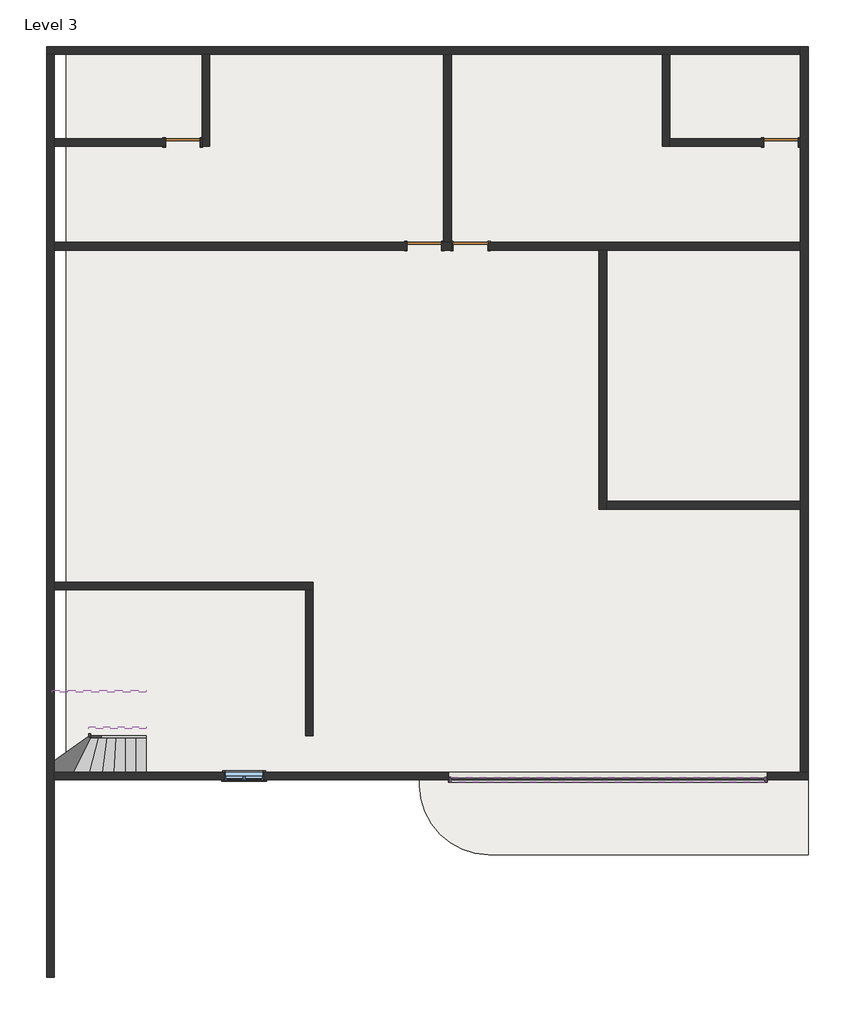
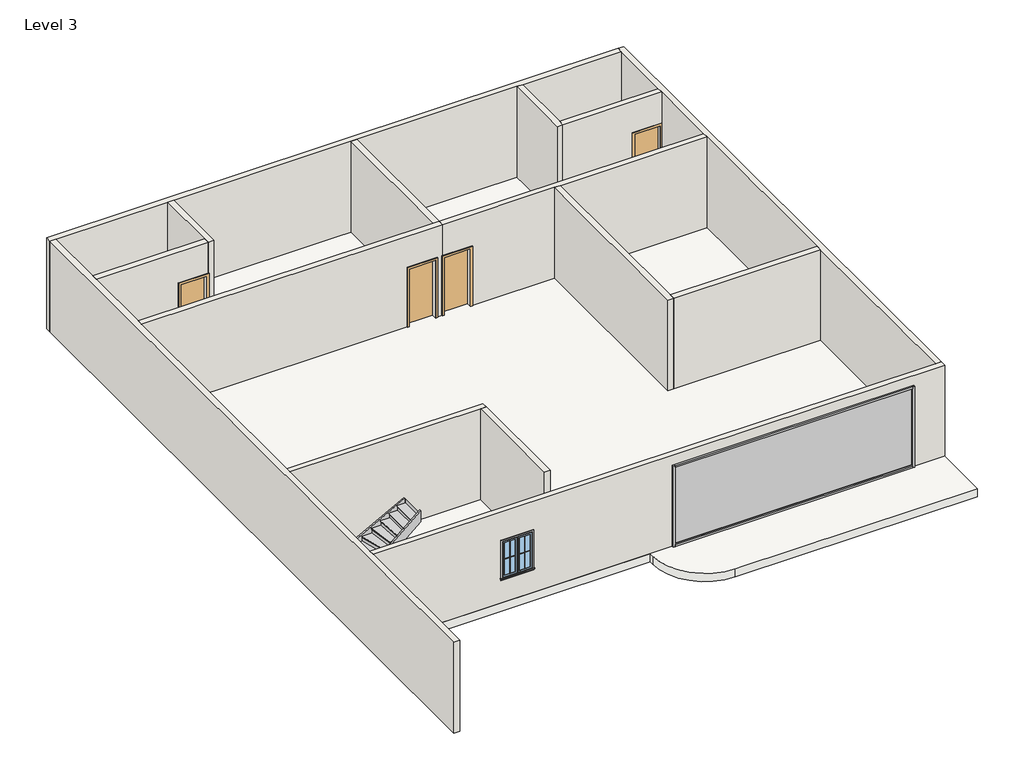
# One storey, incomplete: 15 walls, 12 members, 4 doors, 4 proxies, 1 plate, 1 slab, 1 stair flight, 1 window.
"""IFC4 building model written with IfcOpenShell, lengths in millimetres."""

from ifc_helpers import new_model, si_unit, point, frame, frame_2d, origin, place, context, project, spatial, polyline, circle_curve, trimmed, segment, composite_curve, outline, extrude, faceted_brep, transform, mapped, element, save
from components import muntin_pattern_2x2_muntin_pattern_2x2_88bf7f41, muntin_pattern_2x2_muntin_pattern_2x2_3dfd0a47, trim_window_exterior_flat_with_sill_4930676f, trim_window_interior_flat_picture_frame_dd064338, door_54dd4da4, door_719f80de, member_56b0c076, member_6ded9322, system_panel_glazed_f36121af, stair_flight_a924437b, window_0de3df1e

model = new_model("IFC4")

# Units and contexts
model_context = context("Model", 3, world=origin())
ifc_project = project(units=[si_unit("LENGTHUNIT", "METRE", prefix="MILLI")], contexts=[model_context])

# Site, building, storey
site = spatial("IfcSite", under=ifc_project)
building = spatial("IfcBuilding", under=site)
storey = spatial("IfcBuildingStorey", under=building, Name="Level 3", Elevation=6705.6)

# Proxies
placement = place(None, origin())
muntin_pattern_2x2_muntin_pattern_2x2_shape = muntin_pattern_2x2_muntin_pattern_2x2_88bf7f41(model_context)
element("IfcBuildingElementProxy", 1, Name="Muntin Pattern_2x2 : Muntin Pattern_2x2", ObjectType="Muntin Pattern_2x2 : Muntin Pattern_2x2", at=placement, inside=storey, context=model_context, shape_type="MappedRepresentation", body=[
    mapped(muntin_pattern_2x2_muntin_pattern_2x2_shape, transform((-4862.2306824, -10314.185779, 7689.85), x_axis=(-1.0, 0.0, 0.0), y_axis=(0.0, -1.0, 0.0), z_axis=(0.0, 0.0, 1.0))),
])
muntin_pattern_2x2_muntin_pattern_2x2_2_shape = muntin_pattern_2x2_muntin_pattern_2x2_3dfd0a47(model_context)
element("IfcBuildingElementProxy", 2, Name="Muntin Pattern_2x2 : Muntin Pattern_2x2", ObjectType="Muntin Pattern_2x2 : Muntin Pattern_2x2", at=placement, inside=storey, context=model_context, shape_type="MappedRepresentation", body=[
    mapped(muntin_pattern_2x2_muntin_pattern_2x2_2_shape, transform((-5379.7556824, -10314.185779, 7689.85), x_axis=(1.0, 0.0, 0.0), y_axis=(0.0, 1.0, 0.0), z_axis=(0.0, 0.0, 1.0))),
])
trim_window_exterior_flat_with_sill_shape = trim_window_exterior_flat_with_sill_4930676f(model_context)
element("IfcBuildingElementProxy", 3, Name="Trim-Window-Exterior-Flat : with Sill", ObjectType="Trim-Window-Exterior-Flat : with Sill", at=placement, inside=storey, context=model_context, shape_type="MappedRepresentation", body=[
    mapped(trim_window_exterior_flat_with_sill_shape, transform((-5120.9931824, -10323.710779, 8966.2), x_axis=(1.0, 0.0, 0.0), y_axis=(0.0, 0.0, 1.0), z_axis=(0.0, -1.0, 0.0))),
])
trim_window_interior_flat_picture_frame_shape = trim_window_interior_flat_picture_frame_dd064338(model_context)
element("IfcBuildingElementProxy", 4, Name="Trim-Window-Interior-Flat : Picture Frame", ObjectType="Trim-Window-Interior-Flat : Picture Frame", at=placement, inside=storey, context=model_context, shape_type="MappedRepresentation", body=[
    mapped(trim_window_interior_flat_picture_frame_shape, transform((-5120.9931824, -10120.510779, 8966.2), x_axis=(-1.0, 0.0, 0.0), y_axis=(0.0, 0.0, 1.0), z_axis=(0.0, 1.0, 0.0))),
])

# Doors
door_shape = door_54dd4da4(model_context)
element("IfcDoor", 5, ObjectType="Single-Flush : 36\" x 84\"", at=placement, inside=storey, context=model_context, shape_type="MappedRepresentation", body=[
    mapped(door_shape, transform((-345.7931824, 3798.689221, 6705.6), x_axis=(1.0, 0.0, 0.0), y_axis=(0.0, 1.0, 0.0), z_axis=(0.0, 0.0, 1.0))),
])
element("IfcDoor", 6, ObjectType="Single-Flush : 36\" x 84\"", at=placement, inside=storey, context=model_context, shape_type="MappedRepresentation", body=[
    mapped(door_shape, transform((-6746.5931824, 6541.889221, 6705.6), x_axis=(1.0, 0.0, 0.0), y_axis=(0.0, 1.0, 0.0), z_axis=(0.0, 0.0, 1.0))),
])
door_2_shape = door_719f80de(model_context)
element("IfcDoor", 7, ObjectType="Single-Flush : 36\" x 84\"", at=placement, inside=storey, context=model_context, shape_type="MappedRepresentation", body=[
    mapped(door_2_shape, transform((873.4068176, 3798.689221, 6705.6), x_axis=(-1.0, 0.0, 0.0), y_axis=(0.0, -1.0, 0.0), z_axis=(0.0, 0.0, 1.0))),
])
element("IfcDoor", 8, ObjectType="Single-Flush : 36\" x 84\"", at=placement, inside=storey, context=model_context, shape_type="MappedRepresentation", body=[
    mapped(door_2_shape, transform((9103.0068176, 6541.889221, 6705.6), x_axis=(-1.0, 0.0, 0.0), y_axis=(0.0, -1.0, 0.0), z_axis=(0.0, 0.0, 1.0))),
])

# Members
member_shape = member_56b0c076(model_context)
element("IfcMember", 9, ObjectType="Rectangular Mullion : 2.5\" x 5\" rectangular", at=placement, inside=storey, context=model_context, shape_type="MappedRepresentation", body=[
    mapped(member_shape, transform((296.6565845, -10323.710779, 9700.1946513), x_axis=(-1.0, 0.0, 0.0), y_axis=(0.0, -1.0, 0.0), z_axis=(0.0, 0.0, 1.0))),
])
member_2_shape = member_6ded9322(model_context)
element("IfcMember", 10, ObjectType="Rectangular Mullion : 2.5\" x 5\" rectangular", at=placement, inside=storey, context=model_context, shape_type="MappedRepresentation", body=[
    mapped(member_2_shape, transform((8665.9914897, -10323.710779, 9700.1946513), x_axis=(0.0, 0.0, 1.0), y_axis=(0.0, -1.0, 0.0), z_axis=(1.0, 0.0, 0.0))),
])
element("IfcMember", 11, ObjectType="Rectangular Mullion : 2.5\" x 5\" rectangular", at=placement, inside=storey, context=model_context, shape_type="MappedRepresentation", body=[
    mapped(member_2_shape, transform((360.1565845, -10323.710779, 6705.6), x_axis=(0.0, 0.0, -1.0), y_axis=(0.0, -1.0, 0.0), z_axis=(-1.0, 0.0, 0.0))),
])
element("IfcMember", 12, ObjectType="Rectangular Mullion : 2.5\" x 5\" rectangular", at=placement, inside=storey, context=model_context, shape_type="MappedRepresentation", body=[
    mapped(member_shape, transform((8729.4914897, -10323.710779, 6705.6), x_axis=(1.0, 0.0, 0.0), y_axis=(0.0, -1.0, 0.0), z_axis=(0.0, 0.0, -1.0))),
])
element("IfcMember", 13, ObjectType="Stringer - 2\" Width", at=placement, inside=storey, context=model_context, shape_type="SweptSolid", body=[
    extrude(outline(polyline([(6705.6, -7708.0614906), (6938.0562572, -7708.0614906), (8059.1069249, -9795.4786823), (7713.1321542, -9795.4786823), (6705.6, -7919.4350738), (6705.6, -7708.0614906)])), frame((0.0, -10171.310779, 0.0), z_axis=(0.0, 1.0, 0.0), x_axis=(0.0, 0.0, 1.0)), (0.0, 0.0, 1.0), 50.8),
])
element("IfcMember", 14, ObjectType="Stringer - 2\" Width", at=placement, inside=storey, context=model_context, shape_type="SweptSolid", body=[
    extrude(outline(polyline([(-9795.4786823, -10120.510779), (-9795.4786823, -10171.310779), (-10150.1931824, -10171.310779), (-10150.1931824, -10120.510779), (-9795.4786823, -10120.510779)])), frame((0.0, 0.0, 7713.1321542), z_axis=(0.0, 0.0, 1.0), x_axis=(1.0, 0.0, 0.0)), (0.0, 0.0, 1.0), 345.9747707),
])
element("IfcMember", 15, ObjectType="Stringer - 2\" Width", at=placement, inside=storey, context=model_context, shape_type="SweptSolid", body=[
    extrude(outline(polyline([(-10171.310779, 7754.3069249), (-10171.310779, 8042.1201671), (-8051.2752516, 8751.0282369), (-8012.310779, 8751.0282369), (-8012.310779, 8418.0826013), (-9997.3749587, 7754.3069249), (-10171.310779, 7754.3069249)])), frame((-10200.9931824, 0.0, 0.0), z_axis=(1.0, 0.0, 0.0), x_axis=(0.0, 1.0, 0.0)), (0.0, 0.0, 1.0), 50.8),
])
element("IfcMember", 16, ObjectType="Stringer - 2\" Width", at=placement, inside=storey, context=model_context, shape_type="SweptSolid", body=[
    extrude(outline(polyline([(-10200.9931824, -8012.310779), (-10200.9931824, -7961.510779), (-9795.4786823, -7961.510779), (-9795.4786823, -8012.310779), (-10200.9931824, -8012.310779)])), frame((0.0, 0.0, 8429.6393171), z_axis=(0.0, 0.0, 1.0), x_axis=(1.0, 0.0, 0.0)), (0.0, 0.0, 1.0), 321.3889199),
])
element("IfcMember", 17, ObjectType="Stringer - 2\" Width", at=placement, inside=storey, context=model_context, shape_type="SweptSolid", body=[
    extrude(outline(polyline([(8751.0282369, -9795.4786823), (8429.6393171, -9795.4786823), (9550.6899847, -7708.0614906), (9872.0789046, -7708.0614906), (8751.0282369, -9795.4786823)])), frame((0.0, -8012.310779, 0.0), z_axis=(0.0, 1.0, 0.0), x_axis=(0.0, 0.0, 1.0)), (0.0, 0.0, 1.0), 50.8),
])
element("IfcMember", 18, ObjectType="Stringer - 2\" Width", at=placement, inside=storey, context=model_context, shape_type="SweptSolid", body=[
    extrude(outline(polyline([(6705.6, -7708.0614906), (6883.5241916, -7708.0614906), (8138.4713283, -9184.9931824), (7738.4989166, -9184.9931824), (6705.6, -7969.3872818), (6705.6, -7708.0614906)])), frame((0.0, -9206.110779, 0.0), z_axis=(0.0, 1.0, 0.0), x_axis=(0.0, 0.0, 1.0)), (0.0, 0.0, 1.0), 50.8),
])
element("IfcMember", 19, ObjectType="Stringer - 2\" Width", at=placement, inside=storey, context=model_context, shape_type="SweptSolid", body=[
    extrude(outline(polyline([(-9206.110779, 7781.6636174), (-9206.110779, 8342.1940989), (-9001.0207186, 8707.1714311), (-8977.510779, 8707.1714311), (-8977.510779, 8126.8173278), (-9171.4614414, 7781.6636174), (-9206.110779, 7781.6636174)])), frame((-9235.7931824, 0.0, 0.0), z_axis=(1.0, 0.0, 0.0), x_axis=(0.0, 1.0, 0.0)), (0.0, 0.0, 1.0), 50.8),
])
element("IfcMember", 20, ObjectType="Stringer - 2\" Width", at=placement, inside=storey, context=model_context, shape_type="SweptSolid", body=[
    extrude(outline(polyline([(8707.1714311, -9235.7931824), (8307.1990193, -9235.7931824), (9605.3108568, -7708.0614906), (10005.2832686, -7708.0614906), (8707.1714311, -9235.7931824)])), frame((0.0, -8977.510779, 0.0), z_axis=(0.0, 1.0, 0.0), x_axis=(0.0, 0.0, 1.0)), (0.0, 0.0, 1.0), 50.8),
])

# Plate
system_panel_glazed_shape = system_panel_glazed_f36121af(model_context)
element("IfcPlate", 21, ObjectType="System Panel : Glazed", at=placement, inside=storey, context=model_context, shape_type="MappedRepresentation", body=[
    mapped(system_panel_glazed_shape, transform((4513.0740371, -10323.710779, 6769.1), x_axis=(1.0, 0.0, 0.0), y_axis=(0.0, 1.0, 0.0), z_axis=(0.0, 0.0, 1.0))),
])

# Slab
element("IfcSlab", 22, ObjectType="Generic - 12\"", at=placement, inside=storey, context=model_context, shape_type="SweptSolid", body=[
    extrude(outline(composite_curve([segment(polyline([(-9833.5310626, -10323.710779), (-9833.5310626, 9081.889221), (9814.2068176, 9081.889221), (9814.2068176, -10323.710779), (9814.2068176, -12304.910779), (1356.0068176, -12304.910779)]), True, "CONTINUOUS"), segment(trimmed(circle_curve(frame_2d((1356.0068176, -10476.110779)), 1828.8), [point((1356.0068176, -12304.910779))], [point((-472.7931824, -10476.110779))], False, "CARTESIAN"), True, "CONTINUOUS"), segment(polyline([(-472.7931824, -10476.110779), (-472.7931824, -10323.710779), (-9833.5310626, -10323.710779)]), True, "CONTINUOUS")], self_intersect=False)), frame((0.0, 0.0, 6400.8), z_axis=(0.0, 0.0, 1.0), x_axis=(1.0, 0.0, 0.0)), (0.0, 0.0, 1.0), 304.8),
])

# Stair flight
stair_flight_shape = stair_flight_a924437b(model_context)
element("IfcStairFlight", 23, ObjectType="2\" Tread 1\" Nosing 1/4\" Riser", at=placement, inside=storey, context=model_context, shape_type="MappedRepresentation", body=[
    mapped(stair_flight_shape, transform((0.0, 0.0, 0.0), x_axis=(1.0, 0.0, 0.0), y_axis=(0.0, 1.0, 0.0), z_axis=(0.0, 0.0, 1.0))),
])

# Walls
element("IfcWall", 24, ObjectType="wall.1", at=placement, inside=storey, context=model_context, shape_type="Brep", body=[
    faceted_brep([(-10353.3931824, 8878.689221, 6705.6), (-10150.1931824, 8878.689221, 6705.6), (-6238.5931824, 8878.689221, 6705.6), (-6035.3931824, 8878.689221, 6705.6), (162.2068176, 8878.689221, 6705.6), (365.4068176, 8878.689221, 6705.6), (5953.4068176, 8878.689221, 6705.6), (6156.6068176, 8878.689221, 6705.6), (9611.0068176, 8878.689221, 6705.6), (9611.0068176, 8878.689221, 10058.4), (6156.6068176, 8878.689221, 10058.4), (5953.4068176, 8878.689221, 10058.4), (365.4068176, 8878.689221, 10058.4), (162.2068176, 8878.689221, 10058.4), (-6035.3931824, 8878.689221, 10058.4), (-6238.5931824, 8878.689221, 10058.4), (-10150.1931824, 8878.689221, 10058.4), (-10353.3931824, 8878.689221, 10058.4), (-10353.3931824, 9081.889221, 6705.6), (-10353.3931824, 9081.889221, 10058.4), (9611.0068176, 9081.889221, 10058.4), (9611.0068176, 9081.889221, 6705.6)], [[[0, 1, 2, 3, 4, 5, 6, 7, 8, 9, 10, 11, 12, 13, 14, 15, 16, 17]], [[18, 19, 20, 21]], [[8, 7, 6, 5, 4, 3, 2, 1, 0, 18, 21]], [[17, 16, 15, 14, 13, 12, 11, 10, 9, 20, 19]], [[0, 17, 19, 18]], [[9, 8, 21, 20]]]),
])
element("IfcWall", 25, ObjectType="wall.1", at=placement, inside=storey, context=model_context, shape_type="Brep", body=[
    faceted_brep([(-10150.1931824, -15556.110779, 6705.6), (-10150.1931824, -10323.710779, 6705.6), (-10150.1931824, -10120.510779, 6705.6), (-10150.1931824, -5294.510779, 6705.6), (-10150.1931824, -5091.310779, 6705.6), (-10150.1931824, 3697.089221, 6705.6), (-10150.1931824, 3900.289221, 6705.6), (-10150.1931824, 6440.289221, 6705.6), (-10150.1931824, 6643.489221, 6705.6), (-10150.1931824, 8878.689221, 6705.6), (-10150.1931824, 8878.689221, 10058.4), (-10150.1931824, 6643.489221, 10058.4), (-10150.1931824, 6440.289221, 10058.4), (-10150.1931824, 3900.289221, 10058.4), (-10150.1931824, 3697.089221, 10058.4), (-10150.1931824, -5091.310779, 10058.4), (-10150.1931824, -5294.510779, 10058.4), (-10150.1931824, -10120.510779, 10058.4), (-10150.1931824, -10323.710779, 10058.4), (-10150.1931824, -15556.110779, 10058.4), (-10353.3931824, -15556.110779, 6705.6), (-10353.3931824, -15556.110779, 10058.4), (-10353.3931824, 8878.689221, 10058.4), (-10353.3931824, 8878.689221, 6705.6)], [[[0, 1, 2, 3, 4, 5, 6, 7, 8, 9, 10, 11, 12, 13, 14, 15, 16, 17, 18, 19]], [[20, 21, 22, 23]], [[9, 8, 7, 6, 5, 4, 3, 2, 1, 0, 20, 23]], [[19, 18, 17, 16, 15, 14, 13, 12, 11, 10, 22, 21]], [[0, 19, 21, 20]], [[10, 9, 23, 22]]]),
])
element("IfcWall", 26, ObjectType="wall.1", at=placement, inside=storey, context=model_context, shape_type="Brep", body=[
    faceted_brep([(9814.2068176, -10120.510779, 6705.6), (9611.0068176, -10120.510779, 6705.6), (-10150.1931824, -10120.510779, 6705.6), (-10150.1931824, -10120.510779, 10058.4), (9611.0068176, -10120.510779, 10058.4), (9814.2068176, -10120.510779, 10058.4), (8729.4914897, -10120.510779, 9700.1946513), (296.6565845, -10120.510779, 9700.1946513), (296.6565845, -10120.510779, 6773.2861179), (8729.4914897, -10120.510779, 6773.2861179), (-5641.6931824, -10120.510779, 8966.2), (-5641.6931824, -10120.510779, 7620.0), (-4600.2931824, -10120.510779, 7620.0), (-4600.2931824, -10120.510779, 8966.2), (-10150.1931824, -10323.710779, 6705.6), (9814.2068176, -10323.710779, 6705.6), (9814.2068176, -10323.710779, 10058.4), (-10150.1931824, -10323.710779, 10058.4), (296.6565845, -10323.710779, 9700.1946513), (8729.4914897, -10323.710779, 9700.1946513), (8729.4914897, -10323.710779, 6773.2861179), (296.6565845, -10323.710779, 6773.2861179), (-5641.6931824, -10323.710779, 8966.2), (-4600.2931824, -10323.710779, 8966.2), (-4600.2931824, -10323.710779, 7620.0), (-5641.6931824, -10323.710779, 7620.0)], [[[0, 1, 2, 3, 4, 5], [6, 7, 8, 9], [10, 11, 12, 13]], [[14, 15, 16, 17], [18, 19, 20, 21], [22, 23, 24, 25]], [[2, 1, 0, 15, 14]], [[5, 4, 3, 17, 16]], [[0, 5, 16, 15]], [[6, 19, 18, 7]], [[8, 21, 20, 9]], [[19, 6, 9, 20]], [[7, 18, 21, 8]], [[11, 10, 22, 25]], [[12, 11, 25, 24]], [[13, 12, 24, 23]], [[10, 13, 23, 22]], [[3, 2, 14, 17]]]),
])
element("IfcWall", 27, ObjectType="wall.1", at=placement, inside=storey, context=model_context, shape_type="Brep", body=[
    faceted_brep([(9611.0068176, 9081.889221, 6705.6), (9611.0068176, 8878.689221, 6705.6), (9611.0068176, 6643.489221, 6705.6), (9611.0068176, 6440.289221, 6705.6), (9611.0068176, 3900.289221, 6705.6), (9611.0068176, 3697.089221, 6705.6), (9611.0068176, -2957.710779, 6705.6), (9611.0068176, -3160.910779, 6705.6), (9611.0068176, -10120.510779, 6705.6), (9611.0068176, -10120.510779, 10058.4), (9611.0068176, -3160.910779, 10058.4), (9611.0068176, -2957.710779, 10058.4), (9611.0068176, 3697.089221, 10058.4), (9611.0068176, 3900.289221, 10058.4), (9611.0068176, 6440.289221, 10058.4), (9611.0068176, 6643.489221, 10058.4), (9611.0068176, 8878.689221, 10058.4), (9611.0068176, 9081.889221, 10058.4), (9814.2068176, 9081.889221, 6705.6), (9814.2068176, 9081.889221, 10058.4), (9814.2068176, -10120.510779, 10058.4), (9814.2068176, -10120.510779, 6705.6)], [[[0, 1, 2, 3, 4, 5, 6, 7, 8, 9, 10, 11, 12, 13, 14, 15, 16, 17]], [[18, 19, 20, 21]], [[8, 7, 6, 5, 4, 3, 2, 1, 0, 18, 21]], [[17, 16, 15, 14, 13, 12, 11, 10, 9, 20, 19]], [[0, 17, 19, 18]], [[9, 8, 21, 20]]]),
])
element("IfcWall", 28, ObjectType="wall.1", at=placement, inside=storey, context=model_context, shape_type="SweptSolid", body=[
    extrude(outline(polyline([(162.2068176, 3900.289221), (162.2068176, 8878.689221), (365.4068176, 8878.689221), (365.4068176, 3900.289221), (162.2068176, 3900.289221)])), frame((0.0, 0.0, 6705.6), z_axis=(0.0, 0.0, 1.0), x_axis=(1.0, 0.0, 0.0)), (0.0, 0.0, 1.0), 3352.8),
])
element("IfcWall", 29, ObjectType="wall.1", at=placement, inside=storey, context=model_context, shape_type="Brep", body=[
    faceted_brep([(365.4068176, 3900.289221, 6705.6), (162.2068176, 3900.289221, 6705.6), (111.4068176, 3900.289221, 6705.6), (111.4068176, 3900.289221, 8839.2), (-802.9931824, 3900.289221, 8839.2), (-802.9931824, 3900.289221, 6705.6), (-10150.1931824, 3900.289221, 6705.6), (-10150.1931824, 3900.289221, 10058.4), (162.2068176, 3900.289221, 10058.4), (365.4068176, 3900.289221, 10058.4), (111.4068176, 3697.089221, 8839.2), (111.4068176, 3697.089221, 6705.6), (365.4068176, 3697.089221, 6705.6), (365.4068176, 3697.089221, 10058.4), (-10150.1931824, 3697.089221, 10058.4), (-10150.1931824, 3697.089221, 6705.6), (-802.9931824, 3697.089221, 6705.6), (-802.9931824, 3697.089221, 8839.2)], [[[0, 1, 2, 3, 4, 5, 6, 7, 8, 9]], [[10, 11, 12, 13, 14, 15, 16, 17]], [[16, 15, 6, 5]], [[12, 11, 2, 1, 0]], [[9, 8, 7, 14, 13]], [[7, 6, 15, 14]], [[0, 9, 13, 12]], [[3, 2, 11, 10]], [[4, 3, 10, 17]], [[5, 4, 17, 16]]]),
])
element("IfcWall", 30, ObjectType="wall.1", at=placement, inside=storey, context=model_context, shape_type="Brep", body=[
    faceted_brep([(-6238.5931824, 8878.689221, 6705.6), (-6238.5931824, 6643.489221, 6705.6), (-6238.5931824, 6440.289221, 6705.6), (-6238.5931824, 6440.289221, 10058.4), (-6238.5931824, 6643.489221, 10058.4), (-6238.5931824, 8878.689221, 10058.4), (-6035.3931824, 8878.689221, 6705.6), (-6035.3931824, 8878.689221, 10058.4), (-6035.3931824, 6440.289221, 10058.4), (-6035.3931824, 6440.289221, 6705.6)], [[[0, 1, 2, 3, 4, 5]], [[6, 7, 8, 9]], [[2, 1, 0, 6, 9]], [[5, 4, 3, 8, 7]], [[0, 5, 7, 6]], [[3, 2, 9, 8]]]),
])
element("IfcWall", 31, ObjectType="wall.1", at=placement, inside=storey, context=model_context, shape_type="SweptSolid", body=[
    extrude(outline(polyline([(8839.2, -6289.3931824), (6705.6, -6289.3931824), (6705.6, -6238.5931824), (10058.4, -6238.5931824), (10058.4, -10150.1931824), (6705.6, -10150.1931824), (6705.6, -7203.7931824), (8839.2, -7203.7931824), (8839.2, -6289.3931824)])), frame((0.0, 6440.289221, 0.0), z_axis=(0.0, 1.0, 0.0), x_axis=(0.0, 0.0, 1.0)), (0.0, 0.0, 1.0), 203.2),
])
element("IfcWall", 32, ObjectType="wall.1", at=placement, inside=storey, context=model_context, shape_type="Brep", body=[
    faceted_brep([(365.4068176, 3697.089221, 6705.6), (416.2068176, 3697.089221, 6705.6), (416.2068176, 3697.089221, 8839.2), (1330.6068176, 3697.089221, 8839.2), (1330.6068176, 3697.089221, 6705.6), (4277.0068176, 3697.089221, 6705.6), (4480.2068176, 3697.089221, 6705.6), (9611.0068176, 3697.089221, 6705.6), (9611.0068176, 3697.089221, 10058.4), (4480.2068176, 3697.089221, 10058.4), (4277.0068176, 3697.089221, 10058.4), (365.4068176, 3697.089221, 10058.4), (416.2068176, 3900.289221, 8839.2), (416.2068176, 3900.289221, 6705.6), (365.4068176, 3900.289221, 6705.6), (365.4068176, 3900.289221, 10058.4), (9611.0068176, 3900.289221, 10058.4), (9611.0068176, 3900.289221, 6705.6), (1330.6068176, 3900.289221, 6705.6), (1330.6068176, 3900.289221, 8839.2)], [[[0, 1, 2, 3, 4, 5, 6, 7, 8, 9, 10, 11]], [[12, 13, 14, 15, 16, 17, 18, 19]], [[18, 17, 7, 6, 5, 4]], [[14, 13, 1, 0]], [[11, 10, 9, 8, 16, 15]], [[8, 7, 17, 16]], [[0, 11, 15, 14]], [[2, 1, 13, 12]], [[3, 2, 12, 19]], [[4, 3, 19, 18]]]),
])
element("IfcWall", 33, ObjectType="wall.1", at=placement, inside=storey, context=model_context, shape_type="Brep", body=[
    faceted_brep([(5953.4068176, 8878.689221, 6705.6), (5953.4068176, 6440.289221, 6705.6), (5953.4068176, 6440.289221, 10058.4), (5953.4068176, 8878.689221, 10058.4), (6156.6068176, 8878.689221, 6705.6), (6156.6068176, 8878.689221, 10058.4), (6156.6068176, 6643.489221, 10058.4), (6156.6068176, 6440.289221, 10058.4), (6156.6068176, 6440.289221, 6705.6), (6156.6068176, 6643.489221, 6705.6)], [[[0, 1, 2, 3]], [[4, 5, 6, 7, 8, 9]], [[1, 0, 4, 9, 8]], [[3, 2, 7, 6, 5]], [[0, 3, 5, 4]], [[2, 1, 8, 7]]]),
])
element("IfcWall", 34, ObjectType="wall.1", at=placement, inside=storey, context=model_context, shape_type="SweptSolid", body=[
    extrude(outline(polyline([(6705.6, 6156.6068176), (6705.6, 8645.8068176), (8839.2, 8645.8068176), (8839.2, 9560.2068176), (6705.6, 9560.2068176), (6705.6, 9611.0068176), (10058.4, 9611.0068176), (10058.4, 6156.6068176), (6705.6, 6156.6068176)])), frame((0.0, 6440.289221, 0.0), z_axis=(0.0, 1.0, 0.0), x_axis=(0.0, 0.0, 1.0)), (0.0, 0.0, 1.0), 203.2),
])
element("IfcWall", 35, ObjectType="wall.1", at=placement, inside=storey, context=model_context, shape_type="Brep", body=[
    faceted_brep([(4277.0068176, 3697.089221, 6705.6), (4277.0068176, -3160.910779, 6705.6), (4277.0068176, -3160.910779, 10058.4), (4277.0068176, 3697.089221, 10058.4), (4480.2068176, 3697.089221, 6705.6), (4480.2068176, 3697.089221, 10058.4), (4480.2068176, -2957.710779, 10058.4), (4480.2068176, -3160.910779, 10058.4), (4480.2068176, -3160.910779, 6705.6), (4480.2068176, -2957.710779, 6705.6)], [[[0, 1, 2, 3]], [[4, 5, 6, 7, 8, 9]], [[1, 0, 4, 9, 8]], [[3, 2, 7, 6, 5]], [[0, 3, 5, 4]], [[2, 1, 8, 7]]]),
])
element("IfcWall", 36, ObjectType="wall.1", at=placement, inside=storey, context=model_context, shape_type="SweptSolid", body=[
    extrude(outline(polyline([(9611.0068176, -3160.910779), (4480.2068176, -3160.910779), (4480.2068176, -2957.710779), (9611.0068176, -2957.710779), (9611.0068176, -3160.910779)])), frame((0.0, 0.0, 6705.6), z_axis=(0.0, 0.0, 1.0), x_axis=(1.0, 0.0, 0.0)), (0.0, 0.0, 1.0), 3352.8),
])
element("IfcWall", 37, ObjectType="wall.1", at=placement, inside=storey, context=model_context, shape_type="Brep", body=[
    faceted_brep([(-10150.1931824, -5294.510779, 6705.6), (-3495.3931824, -5294.510779, 6705.6), (-3292.1931824, -5294.510779, 6705.6), (-3292.1931824, -5294.510779, 10058.4), (-3495.3931824, -5294.510779, 10058.4), (-10150.1931824, -5294.510779, 10058.4), (-10150.1931824, -5091.310779, 6705.6), (-10150.1931824, -5091.310779, 10058.4), (-3292.1931824, -5091.310779, 10058.4), (-3292.1931824, -5091.310779, 6705.6)], [[[0, 1, 2, 3, 4, 5]], [[6, 7, 8, 9]], [[2, 1, 0, 6, 9]], [[5, 4, 3, 8, 7]], [[0, 5, 7, 6]], [[3, 2, 9, 8]]]),
])
element("IfcWall", 38, ObjectType="wall.1", at=placement, inside=storey, context=model_context, shape_type="SweptSolid", body=[
    extrude(outline(polyline([(-3495.3931824, -9155.310779), (-3495.3931824, -5294.510779), (-3292.1931824, -5294.510779), (-3292.1931824, -9155.310779), (-3495.3931824, -9155.310779)])), frame((0.0, 0.0, 6705.6), z_axis=(0.0, 0.0, 1.0), x_axis=(1.0, 0.0, 0.0)), (0.0, 0.0, 1.0), 3352.8),
])

# Window
window_shape = window_0de3df1e(model_context)
element("IfcWindow", 39, ObjectType="Window-Casement-Double : 41\" x 53\"", at=placement, inside=storey, context=model_context, shape_type="MappedRepresentation", body=[
    mapped(window_shape, transform((-5120.9931824, -10222.110779, 6705.6), x_axis=(-1.0, 0.0, 0.0), y_axis=(0.0, -1.0, 0.0), z_axis=(0.0, 0.0, 1.0))),
])

save(model, "model.ifc")

# Revit data of these elements
# Type "Muntin Pattern_2x2 : Muntin Pattern_2x2"
#   Width [instance default] = 4' - 0"
#   Thickness = 0' - 0 1/2"
#   Height [instance default] = 4' - 0"
#   Distance = 0' - 0 3/4"
#   Interior Material [instance default] = none
#   Exterior Material [instance default] = none
#   Default Elevation = 0
# Type "Trim-Window-Exterior-Flat : with Sill"
#   Trim Width = 0' - 2 1/4"
#   Trim Thickness_Picture Frame = 0' - 1 1/4"
#   Trim Thickness_with Sill = 0' - 0 3/4"
#   Sill Thickness = 0' - 1 1/4"
#   Opening Width [instance default] = 2' - 0"
#   Opening Height [instance default] = 3' - 0"
#   Default Elevation = 4' - 0"
#   Sill = yes
#   Picture Frame = no
#   Trim Material [instance default] = none
# Type "Trim-Window-Interior-Flat : Picture Frame"
#   Trim Thickness_Picture Frame = 0' - 1 1/4"
#   Trim Width = 0' - 2 1/4"
#   Trim Thickness_with Sill = 0' - 0 3/4"
#   Sill Thickness = 0' - 1 1/4"
#   Opening Width [instance default] = 2' - 0"
#   Opening Height [instance default] = 3' - 0"
#   Default Elevation = 4' - 0"
#   Sill = no
#   Picture Frame = yes
#   Trim Material [instance default] = none
# Type "Single-Flush : 36\" x 84\""
#   Type Mark = "1"
#   Construction Type Id = "MDOOR"
#   Assembly Code = "C1020"
#   Analytic Construction = "Metal"
#   Thickness = 0' - 2"
#   Heat Transfer Coefficient (U) = 0.651978 BTU/(h·ft²·°F)
#   Height = 7' - 0"
#   Trim Projection Ext = 0' - 1"
#   Trim Projection Int = 0' - 1"
#   Trim Width = 0' - 3"
#   Width = 3' - 0"
#   Define Thermal Properties by = 1
#   Define Thermal Properties by = 1
#   Door Material = Door - Panel
#   Frame Material = Door - Frame
#   Visual Light Transmittance = 0
#   Solar Heat Gain Coefficient = 0
#   Function = (empty or 0)
#   Wall Closure = (empty or 0)
# Type "Rectangular Mullion : 2.5\" x 5\" rectangular"
#   built-in parameter 1007304 = 0.416667 (stored number, unit not read)
#   built-in parameter 1007301 = 0.104167 (stored number, unit not read)
#   built-in parameter 1007300 = 0.104167 (stored number, unit not read)
# Type "System Panel : Glazed"
#   Construction Type Id = "GSP4R"
#   Analytic Construction = "1/8 in Pilkington single glazing"
#   Visual Light Transmittance = 0.9
#   Solar Heat Gain Coefficient = 0.86
#   Heat Transfer Coefficient (U) = 1.18115 BTU/(h·ft²·°F)
#   Define Thermal Properties by = 1
# Type "Generic - 12\""
#   Assembly Code = "B1010"
#   Function = 0
#   Layers, outside or top first: 1' - 0" no material (function 1)
# Type "wall.1"
#   Assembly Code = "B2010"
#   Layers, outside or top first: 0' - 8" no material (function 1)
# Type "Window-Casement-Double : 41\" x 53\""
#   Type Mark = "15"
#   Fire Rating = "0.5h"
#   Assembly Code = "B2020100"
#   Analytic Construction = "Double glazing - domestic"
#   Frame Extension [instance default] = 0' - 0 1/4"
#   Window Inset [instance default] = 0' - 0"
#   Wall Thickness [instance default] = 0' - 6"
#   Interior Wall Closure [instance default] = 0' - 2 1/4"
#   Half Width = 1' - 8 1/2"
#   Visual Light Transmittance = 0.81
#   Thermal Resistance (R) = 1.8146 (h·ft²·°F)/BTU
#   Solar Heat Gain Coefficient = 0.76
#   Rough Width = 3' - 5 1/2"
#   Rough Height = 4' - 5 1/2"
#   Height = 4' - 5"
#   Heat Transfer Coefficient (U) = 0.5511 BTU/(h·ft²·°F)
#   Exterior Wall Closure [instance default] = 0' - 1 1/4"
#   Extension Jamb [instance default] = 0' - 2 1/4"
#   Default Sill Height = 3' - 0"
#   Width = 3' - 5"
#   Define Thermal Properties by = 0
#   Muntin Visibility = yes
#   Interior Trim Visibility [instance default] = yes
#   Exterior Trim Visibility [instance default] = yes
#   Extension Jamb Visibility [instance default] = yes
#   Interior Trim Material = Wood - Stained
#   Muntin Pattern = Muntin Pattern_2x2 : Muntin Pattern_2x2
#   Interior Trim = Trim-Window-Interior-Flat : Picture Frame
#   Interior Frame Material = Wood - Stained
#   Glass Panel Material = Glass
#   Exterior Trim Material = Clad - White
#   Exterior Trim = Trim-Window-Exterior-Flat : with Sill
#   Exterior Frame Material = Clad - White
#   Wall Closure = (empty or 0)
# Elements 1, 2 (IfcBuildingElementProxy, "Muntin Pattern_2x2 : Muntin Pattern_2x2")
#   Width = 1' - 3 1/8"
#   Height = 3' - 11 1/2"
#   Interior Material = Wood - Stained
#   Exterior Material = Clad - White
#   Phase Created = New Construction
#   Materials on its faces: "Clad - White", "Wood - Stained"
# Element 3 (IfcBuildingElementProxy, "Trim-Window-Exterior-Flat : with Sill")
#   Opening Width = 3' - 5"
#   Opening Height = 4' - 5"
#   Trim Material = Clad - White
#   Phase Created = New Construction
#   Materials on its faces: "Clad - White"
# Element 4 (IfcBuildingElementProxy, "Trim-Window-Interior-Flat : Picture Frame")
#   Opening Width = 3' - 5"
#   Opening Height = 4' - 5"
#   Trim Material = Wood - Stained
#   Phase Created = New Construction
#   Materials on its faces: "Wood - Stained"
# Elements 5, 6, 7, 8 (IfcDoor, "Single-Flush : 36\" x 84\"")
#   Phase Created = New Construction
#   Materials on its faces: "Door - Frame", "Door - Panel"
# Elements 9, 10, 11, 12 (IfcMember, "Rectangular Mullion : 2.5\" x 5\" rectangular")
#   Phase Created = New Construction
#   Materials on its faces: "Aluminum"
# Elements 13, 14, 15, 16, 17, 18, 19, 20 (IfcMember, "Stringer - 2\" Width")
#   Phase Created = New Construction
# Element 21 (IfcPlate, "System Panel : Glazed")
#   Phase Created = New Construction
#   Materials on its faces: "Glass"
# Element 22 (IfcSlab, "Generic - 12\"")
#   built-in parameter 1001955 = -1.5708 (stored number, unit not read)
#   Height Offset From Level = 0' - 0"
#   Phase Created = New Construction
#   Materials on its faces: "Default Floor", "LL", "BLUE", "GHT"
# Element 23 (IfcStairFlight, "2\" Tread 1\" Nosing 1/4\" Riser")
#   Phase Created = New Construction
# Elements 24, 25, 26, 27 (IfcWall, "wall.1")
#   Top Offset = 0' - 0"
#   Base Offset = 0' - 0"
#   Unconnected Height = 11' - 0"
#   wall height = 11' - 0"
#   Phase Created = New Construction
#   Base Constraint = Level 3
#   Materials on its faces: "Default Wall", "GHT"
# Elements 28, 29, 30, 31, 32, 33, 34, 35, 36, 38 (IfcWall, "wall.1")
#   Top Offset = 0' - 0"
#   Base Offset = 0' - 0"
#   Unconnected Height = 11' - 0"
#   wall height = 11' - 0"
#   Phase Created = New Construction
#   Base Constraint = Level 3
#   Materials on its faces: "Default Wall"
# Element 37 (IfcWall, "wall.1")
#   Top Offset = 0' - 0"
#   Base Offset = 0' - 0"
#   Unconnected Height = 11' - 0"
#   wall height = 11' - 0"
#   Phase Created = New Construction
#   Base Constraint = Level 3
#   Materials on its faces: "Default Wall", "Softwood, Lumber"
# Element 39 (IfcWindow, "Window-Casement-Double : 41\" x 53\"")
#   Mark = "3"
#   Window Inset = 0' - 0"
#   Interior Wall Closure = 0' - 2 1/4"
#   Frame Extension = 0' - 0 1/4"
#   Exterior Wall Closure = 0' - 1 1/4"
#   Interior Trim Visibility = yes
#   Exterior Trim Visibility = yes
#   Phase Created = New Construction
#   Materials on its faces: "Wood - Stained", "Glass", "Clad - White"
# Materials
#   "Door - Panel": class "Wood", colour RGB 210 159 95, transparency 0, Cost = 0
#   "Door - Frame": colour RGB 118 70 51, transparency 0, Cost = 0
#   "Wood - Stained": class "Wood", colour RGB 224 178 126, transparency 0, Cost = 0
#   "Glass": class "Glass", colour RGB 0 128 192, transparency 0.75, Description = "Soda Lime Glass", Cost = 0
#   "Clad - White": class "Wood", colour RGB 242 242 238, transparency 0, Cost = 0
#   "Aluminum": class "Metal", colour RGB 247 247 247, transparency 0, Description = "Aluminum 6061", Cost = 0
#   "Default Floor": colour RGB 128 128 128, transparency 0, Cost = 0
#   "LL": class "Generic", colour RGB 120 120 120, transparency 0, Cost = 0
#   "BLUE": class "Generic", colour RGB 120 120 120, transparency 0, Cost = 0
#   "GHT": class "Generic", colour RGB 120 120 120, transparency 0, Cost = 0
#   "Default Wall": colour RGB 128 128 128, transparency 0, Cost = 0
#   "Softwood, Lumber": class "Wood", colour RGB 223 192 134, transparency 0, Description = "Pinus Echinata", Cost = 0
